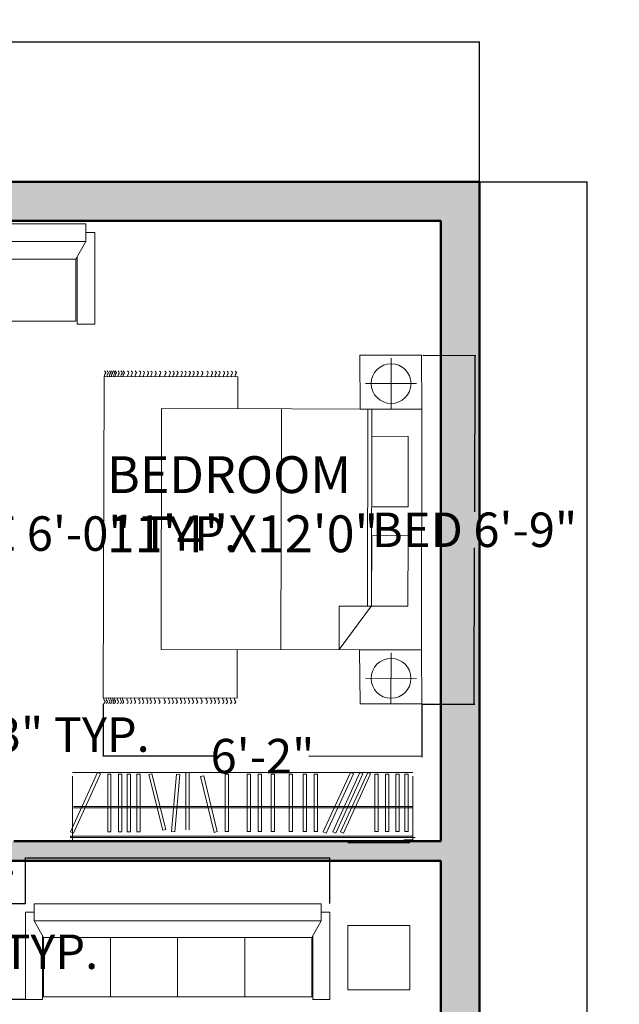
# Model space of a CAD drawing. Units: inches. Extents: x 22042254 to 25404563, y 17568978 to 17626777.
# Tile 44 of 45: x 22180037 to 22180176, y 17626547 to 17626775. Entities that reach past the tile are written whole.
import ezdxf

# ---------------------------------------------------------------- set-up
doc = ezdxf.new("R2010")
doc.units = ezdxf.units.IN
doc.header["$MEASUREMENT"] = 0
for name, color, linetype, lineweight in [('A-ANNO-DIMS', 2, 'Continuous', 18), ('A-AREA-IDEN', 7, 'Continuous', 18), ('A-WALL-PATT', 244, 'Continuous', 13), ('closet', 252, 'Continuous', 18), ('furniture', 8, 'Continuous', 18), ('walls', 252, 'Continuous', 50)]:
    doc.layers.add(name, color=color, linetype=linetype, lineweight=lineweight)
doc.styles.get("Standard").update_dxf_attribs({"font": 'arial.ttf'})
doc.dimstyles.get("Standard").update_dxf_attribs({"dimtxt": 8, "dimasz": 0.18, "dimexe": 0.18, "dimexo": 0.0625, "dimgap": 0.09, "dimtad": 0, "dimtih": 1, "dimtoh": 1, "dimzin": 0, "dimdsep": 46, "dimlunit": 3, "dimtxsty": 'Standard', "dimcen": 0.09, "dimadec": 0, "dimazin": 0, "dimtfac": 1, "dimtofl": 0, "dimtmove": 0, "dimatfit": 3, "dimfxl": 1, "dimtolj": 1, "dimtzin": 0, "dimarcsym": 0})

# ---------------------------------------------------------------- blocks, each defined once
blk = doc.blocks.new('*D1')
at = {"layer": 'A-ANNO-DIMS', "color": 0, "lineweight": -2, "transparency": 16777216}
for p, q in [((22179783.73, 17626737.84), (22179783.73, 17626770.35)), ((22179783.91, 17626770.17), (22179956.86, 17626770.17)), ((22180143.55, 17626770.17), (22179970.61, 17626770.17)), ((22180143.73, 17626737.84), (22180143.73, 17626770.35))]:
    blk.add_line(p, q, dxfattribs=at)
at = {"layer": 'A-ANNO-DIMS', "color": 0, "transparency": 16777216}
for points in [[(22179783.91, 17626770.2), (22179783.91, 17626770.14), (22179783.73, 17626770.17)], [(22180143.55, 17626770.2), (22180143.55, 17626770.14), (22180143.73, 17626770.17)]]:
    blk.add_solid(points, dxfattribs=at)
at = {"layer": 'Defpoints', "color": 0, "transparency": 16777216}
for p in [(22180143.73, 17626770.17), (22179783.73, 17626737.78), (22180143.73, 17626737.78)]:
    blk.add_point(p, dxfattribs=at)
at = {"layer": 'A-ANNO-DIMS', "color": 0, "transparency": 16777216, "insert": (22179963.73, 17626770.17), "char_height": 8, "attachment_point": 5}
blk.add_mtext("\\A1;30'", dxfattribs=at)
blk = doc.blocks.new('*D2')
at = {"layer": 'A-ANNO-DIMS', "color": 0, "lineweight": -2, "transparency": 16777216}
for p, q in [((22180143.8, 17626737.78), (22180168.82, 17626737.78)), ((22180168.64, 17626737.6), (22180168.64, 17626471.94)), ((22180168.64, 17626197.96), (22180168.64, 17626463.62)), ((22180143.8, 17626197.78), (22180168.82, 17626197.78))]:
    blk.add_line(p, q, dxfattribs=at)
at = {"layer": 'A-ANNO-DIMS', "color": 0, "transparency": 16777216}
for points in [[(22180168.61, 17626737.6), (22180168.67, 17626737.6), (22180168.64, 17626737.78)], [(22180168.61, 17626197.96), (22180168.67, 17626197.96), (22180168.64, 17626197.78)]]:
    blk.add_solid(points, dxfattribs=at)
at = {"layer": 'Defpoints', "color": 0, "transparency": 16777216}
for p in [(22180143.73, 17626737.78), (22180168.64, 17626737.78), (22180143.73, 17626197.78)]:
    blk.add_point(p, dxfattribs=at)
at = {"layer": 'A-ANNO-DIMS', "color": 0, "transparency": 16777216, "insert": (22180168.64, 17626467.78), "char_height": 8, "attachment_point": 5}
blk.add_mtext("\\A1;45'", dxfattribs=at)
blk = doc.blocks.new('FABRIC SOFA 4S')
at = {"layer": 'furniture'}
for p, q in [((3, 54), (34, 54)), ((3, 51), (3, 54)), ((34, 48), (34, 54)), ((0, -51), (0, 51)), ((6, 51), (0, 51)), ((6, -51), (6, 51)), ((12, 47.63), (6, 51)), ((11.14, 48), (34, 48)), ((33, 23.81), (12, 23.81)), ((33, 0), (12, 0)), ((33, -23.81), (12, -23.81)), ((6, -51), (12, -47.63)), ((11.54, -48), (34, -48)), ((34, -48), (34, -54)), ((6, -51), (0, -51)), ((3, -54), (3, -51)), ((3, -54), (34, -54))]:
    blk.add_line(p, q, dxfattribs=at)
blk.add_lwpolyline([(12, -47.63), (12, 47.63), (33, 47.63), (33, -47.63)], close=True, dxfattribs=at)
blk = doc.blocks.new('CARPET')
at = {"layer": 'furniture'}
for p, q in [((-51.53, -98.11), (-51.53, -55.12)), ((-51.53, -55.12), (-41.27, -55.12)), ((36, -55.12), (51.55, -55.12)), ((51.55, -55.12), (51.55, -98.11)), ((51.55, -98.11), (-51.53, -98.11))]:
    blk.add_line(p, q, dxfattribs=at)
for points, knots in [([(-53.37, -55.99), (-53.22, -55.8), (-52.9, -55.41), (-52.34, -55.8), (-51.89, -56.08), (-51.65, -55.91), (-51.53, -55.83)], [0, 0, 0, 0, 0.653278, 1.290138, 1.740457, 2.114451, 2.114451, 2.114451, 2.114451]), ([(-53.37, -57.26), (-53.22, -57.07), (-52.9, -56.67), (-52.34, -57.07), (-51.89, -57.35), (-51.65, -57.17), (-51.53, -57.1)], [0, 0, 0, 0, 0.653278, 1.290138, 1.740457, 2.114451, 2.114451, 2.114451, 2.114451]), ([(53.37, -55.99), (53.22, -55.8), (52.9, -55.41), (52.34, -55.8), (51.89, -56.08), (51.65, -55.91), (51.53, -55.83)], [0, 0, 0, 0, 0.653278, 1.290138, 1.740457, 2.114451, 2.114451, 2.114451, 2.114451]), ([(53.37, -57.26), (53.22, -57.07), (52.9, -56.67), (52.34, -57.07), (51.89, -57.35), (51.65, -57.17), (51.53, -57.1)], [0, 0, 0, 0, 0.653278, 1.290138, 1.740457, 2.114451, 2.114451, 2.114451, 2.114451]), ([(-53.37, -58.59), (-53.22, -58.4), (-52.9, -58.01), (-52.34, -58.4), (-51.89, -58.68), (-51.65, -58.5), (-51.53, -58.43)], [0, 0, 0, 0, 0.653278, 1.290138, 1.740457, 2.114451, 2.114451, 2.114451, 2.114451]), ([(-53.37, -59.78), (-53.22, -59.58), (-52.9, -59.19), (-52.34, -59.58), (-51.89, -59.86), (-51.65, -59.69), (-51.53, -59.61)], [0, 0, 0, 0, 0.653278, 1.290138, 1.740457, 2.114451, 2.114451, 2.114451, 2.114451]), ([(53.37, -58.59), (53.22, -58.4), (52.9, -58.01), (52.34, -58.4), (51.89, -58.68), (51.65, -58.5), (51.53, -58.43)], [0, 0, 0, 0, 0.653278, 1.290138, 1.740457, 2.114451, 2.114451, 2.114451, 2.114451]), ([(53.37, -59.78), (53.22, -59.58), (52.9, -59.19), (52.34, -59.58), (51.89, -59.86), (51.65, -59.69), (51.53, -59.61)], [0, 0, 0, 0, 0.653278, 1.290138, 1.740457, 2.114451, 2.114451, 2.114451, 2.114451]), ([(-53.37, -61.22), (-53.22, -61.02), (-52.9, -60.63), (-52.34, -61.02), (-51.89, -61.3), (-51.65, -61.13), (-51.53, -61.05)], [0, 0, 0, 0, 0.653278, 1.290138, 1.740457, 2.114451, 2.114451, 2.114451, 2.114451]), ([(-53.37, -62.44), (-53.22, -62.25), (-52.9, -61.86), (-52.34, -62.25), (-51.89, -62.53), (-51.65, -62.36), (-51.53, -62.28)], [0, 0, 0, 0, 0.653278, 1.290138, 1.740457, 2.114451, 2.114451, 2.114451, 2.114451]), ([(-53.37, -63.63), (-53.22, -63.43), (-52.9, -63.04), (-52.34, -63.43), (-51.89, -63.72), (-51.65, -63.54), (-51.53, -63.46)], [0, 0, 0, 0, 0.653278, 1.290138, 1.740457, 2.114451, 2.114451, 2.114451, 2.114451]), ([(53.37, -61.22), (53.22, -61.02), (52.9, -60.63), (52.34, -61.02), (51.89, -61.3), (51.65, -61.13), (51.53, -61.05)], [0, 0, 0, 0, 0.653278, 1.290138, 1.740457, 2.114451, 2.114451, 2.114451, 2.114451]), ([(53.37, -62.44), (53.22, -62.25), (52.9, -61.86), (52.34, -62.25), (51.89, -62.53), (51.65, -62.36), (51.53, -62.28)], [0, 0, 0, 0, 0.653278, 1.290138, 1.740457, 2.114451, 2.114451, 2.114451, 2.114451]), ([(53.37, -63.63), (53.22, -63.43), (52.9, -63.04), (52.34, -63.43), (51.89, -63.72), (51.65, -63.54), (51.53, -63.46)], [0, 0, 0, 0, 0.653278, 1.290138, 1.740457, 2.114451, 2.114451, 2.114451, 2.114451]), ([(-53.37, -65.07), (-53.22, -64.87), (-52.9, -64.48), (-52.34, -64.87), (-51.89, -65.15), (-51.65, -64.98), (-51.53, -64.9)], [0, 0, 0, 0, 0.653278, 1.290138, 1.740457, 2.114451, 2.114451, 2.114451, 2.114451]), ([(-53.37, -66.76), (-53.22, -66.56), (-52.9, -66.17), (-52.34, -66.56), (-51.89, -66.84), (-51.65, -66.67), (-51.53, -66.59)], [0, 0, 0, 0, 0.653278, 1.290138, 1.740457, 2.114451, 2.114451, 2.114451, 2.114451]), ([(53.37, -65.07), (53.22, -64.87), (52.9, -64.48), (52.34, -64.87), (51.89, -65.15), (51.65, -64.98), (51.53, -64.9)], [0, 0, 0, 0, 0.653278, 1.290138, 1.740457, 2.114451, 2.114451, 2.114451, 2.114451]), ([(53.37, -66.76), (53.22, -66.56), (52.9, -66.17), (52.34, -66.56), (51.89, -66.84), (51.65, -66.67), (51.53, -66.59)], [0, 0, 0, 0, 0.653278, 1.290138, 1.740457, 2.114451, 2.114451, 2.114451, 2.114451]), ([(-53.37, -68.2), (-53.22, -68), (-52.9, -67.61), (-52.34, -68), (-51.89, -68.28), (-51.65, -68.11), (-51.53, -68.03)], [0, 0, 0, 0, 0.653278, 1.290138, 1.740457, 2.114451, 2.114451, 2.114451, 2.114451]), ([(-53.37, -69.53), (-53.22, -69.33), (-52.9, -68.94), (-52.34, -69.33), (-51.89, -69.61), (-51.65, -69.44), (-51.53, -69.36)], [0, 0, 0, 0, 0.653278, 1.290138, 1.740457, 2.114451, 2.114451, 2.114451, 2.114451]), ([(53.37, -68.2), (53.22, -68), (52.9, -67.61), (52.34, -68), (51.89, -68.28), (51.65, -68.11), (51.53, -68.03)], [0, 0, 0, 0, 0.653278, 1.290138, 1.740457, 2.114451, 2.114451, 2.114451, 2.114451]), ([(53.37, -69.53), (53.22, -69.33), (52.9, -68.94), (52.34, -69.33), (51.89, -69.61), (51.65, -69.44), (51.53, -69.36)], [0, 0, 0, 0, 0.653278, 1.290138, 1.740457, 2.114451, 2.114451, 2.114451, 2.114451]), ([(-53.37, -70.79), (-53.22, -70.6), (-52.9, -70.21), (-52.34, -70.6), (-51.89, -70.88), (-51.65, -70.7), (-51.53, -70.63)], [0, 0, 0, 0, 0.653278, 1.290138, 1.740457, 2.114451, 2.114451, 2.114451, 2.114451]), ([(-53.37, -72.12), (-53.22, -71.93), (-52.9, -71.54), (-52.34, -71.93), (-51.89, -72.21), (-51.65, -72.04), (-51.53, -71.96)], [0, 0, 0, 0, 0.653278, 1.290138, 1.740457, 2.114451, 2.114451, 2.114451, 2.114451]), ([(53.37, -70.79), (53.22, -70.6), (52.9, -70.21), (52.34, -70.6), (51.89, -70.88), (51.65, -70.7), (51.53, -70.63)], [0, 0, 0, 0, 0.653278, 1.290138, 1.740457, 2.114451, 2.114451, 2.114451, 2.114451]), ([(53.37, -72.12), (53.22, -71.93), (52.9, -71.54), (52.34, -71.93), (51.89, -72.21), (51.65, -72.04), (51.53, -71.96)], [0, 0, 0, 0, 0.653278, 1.290138, 1.740457, 2.114451, 2.114451, 2.114451, 2.114451]), ([(-53.37, -73.31), (-53.22, -73.11), (-52.9, -72.72), (-52.34, -73.11), (-51.89, -73.4), (-51.65, -73.22), (-51.53, -73.14)], [0, 0, 0, 0, 0.653278, 1.290138, 1.740457, 2.114451, 2.114451, 2.114451, 2.114451]), ([(-53.37, -74.75), (-53.22, -74.55), (-52.9, -74.16), (-52.34, -74.55), (-51.89, -74.83), (-51.65, -74.66), (-51.53, -74.58)], [0, 0, 0, 0, 0.653278, 1.290138, 1.740457, 2.114451, 2.114451, 2.114451, 2.114451]), ([(-53.37, -75.98), (-53.22, -75.78), (-52.9, -75.39), (-52.34, -75.78), (-51.89, -76.06), (-51.65, -75.89), (-51.53, -75.81)], [0, 0, 0, 0, 0.653278, 1.290138, 1.740457, 2.114451, 2.114451, 2.114451, 2.114451]), ([(53.37, -73.31), (53.22, -73.11), (52.9, -72.72), (52.34, -73.11), (51.89, -73.4), (51.65, -73.22), (51.53, -73.14)], [0, 0, 0, 0, 0.653278, 1.290138, 1.740457, 2.114451, 2.114451, 2.114451, 2.114451]), ([(53.37, -74.75), (53.22, -74.55), (52.9, -74.16), (52.34, -74.55), (51.89, -74.83), (51.65, -74.66), (51.53, -74.58)], [0, 0, 0, 0, 0.653278, 1.290138, 1.740457, 2.114451, 2.114451, 2.114451, 2.114451]), ([(53.37, -75.98), (53.22, -75.78), (52.9, -75.39), (52.34, -75.78), (51.89, -76.06), (51.65, -75.89), (51.53, -75.81)], [0, 0, 0, 0, 0.653278, 1.290138, 1.740457, 2.114451, 2.114451, 2.114451, 2.114451]), ([(-53.37, -77.16), (-53.22, -76.96), (-52.9, -76.57), (-52.34, -76.96), (-51.89, -77.25), (-51.65, -77.07), (-51.53, -76.99)], [0, 0, 0, 0, 0.653278, 1.290138, 1.740457, 2.114451, 2.114451, 2.114451, 2.114451]), ([(-53.37, -78.6), (-53.22, -78.4), (-52.9, -78.01), (-52.34, -78.4), (-51.89, -78.68), (-51.65, -78.51), (-51.53, -78.43)], [0, 0, 0, 0, 0.653278, 1.290138, 1.740457, 2.114451, 2.114451, 2.114451, 2.114451]), ([(53.37, -77.16), (53.22, -76.96), (52.9, -76.57), (52.34, -76.96), (51.89, -77.25), (51.65, -77.07), (51.53, -76.99)], [0, 0, 0, 0, 0.653278, 1.290138, 1.740457, 2.114451, 2.114451, 2.114451, 2.114451]), ([(53.37, -78.6), (53.22, -78.4), (52.9, -78.01), (52.34, -78.4), (51.89, -78.68), (51.65, -78.51), (51.53, -78.43)], [0, 0, 0, 0, 0.653278, 1.290138, 1.740457, 2.114451, 2.114451, 2.114451, 2.114451]), ([(-53.37, -80.29), (-53.22, -80.09), (-52.9, -79.7), (-52.34, -80.09), (-51.89, -80.37), (-51.65, -80.2), (-51.53, -80.12)], [0, 0, 0, 0, 0.653278, 1.290138, 1.740457, 2.114451, 2.114451, 2.114451, 2.114451]), ([(-53.37, -81.73), (-53.22, -81.53), (-52.9, -81.14), (-52.34, -81.53), (-51.89, -81.81), (-51.65, -81.64), (-51.53, -81.56)], [0, 0, 0, 0, 0.653278, 1.290138, 1.740457, 2.114451, 2.114451, 2.114451, 2.114451]), ([(53.37, -80.29), (53.22, -80.09), (52.9, -79.7), (52.34, -80.09), (51.89, -80.37), (51.65, -80.2), (51.53, -80.12)], [0, 0, 0, 0, 0.653278, 1.290138, 1.740457, 2.114451, 2.114451, 2.114451, 2.114451]), ([(53.37, -81.73), (53.22, -81.53), (52.9, -81.14), (52.34, -81.53), (51.89, -81.81), (51.65, -81.64), (51.53, -81.56)], [0, 0, 0, 0, 0.653278, 1.290138, 1.740457, 2.114451, 2.114451, 2.114451, 2.114451]), ([(-53.37, -83.06), (-53.22, -82.86), (-52.9, -82.47), (-52.34, -82.86), (-51.89, -83.14), (-51.65, -82.97), (-51.53, -82.89)], [0, 0, 0, 0, 0.653278, 1.290138, 1.740457, 2.114451, 2.114451, 2.114451, 2.114451]), ([(-53.37, -84.18), (-53.22, -83.99), (-52.9, -83.6), (-52.34, -83.99), (-51.89, -84.27), (-51.65, -84.09), (-51.53, -84.02)], [0, 0, 0, 0, 0.653278, 1.290138, 1.740457, 2.114451, 2.114451, 2.114451, 2.114451]), ([(-53.37, -85.51), (-53.22, -85.32), (-52.9, -84.93), (-52.34, -85.32), (-51.89, -85.6), (-51.65, -85.42), (-51.53, -85.35)], [0, 0, 0, 0, 0.653278, 1.290138, 1.740457, 2.114451, 2.114451, 2.114451, 2.114451]), ([(53.37, -83.06), (53.22, -82.86), (52.9, -82.47), (52.34, -82.86), (51.89, -83.14), (51.65, -82.97), (51.53, -82.89)], [0, 0, 0, 0, 0.653278, 1.290138, 1.740457, 2.114451, 2.114451, 2.114451, 2.114451]), ([(53.37, -84.18), (53.22, -83.99), (52.9, -83.6), (52.34, -83.99), (51.89, -84.27), (51.65, -84.09), (51.53, -84.02)], [0, 0, 0, 0, 0.653278, 1.290138, 1.740457, 2.114451, 2.114451, 2.114451, 2.114451]), ([(53.37, -85.51), (53.22, -85.32), (52.9, -84.93), (52.34, -85.32), (51.89, -85.6), (51.65, -85.42), (51.53, -85.35)], [0, 0, 0, 0, 0.653278, 1.290138, 1.740457, 2.114451, 2.114451, 2.114451, 2.114451]), ([(-53.37, -86.7), (-53.22, -86.5), (-52.9, -86.11), (-52.34, -86.5), (-51.89, -86.78), (-51.65, -86.61), (-51.53, -86.53)], [0, 0, 0, 0, 0.653278, 1.290138, 1.740457, 2.114451, 2.114451, 2.114451, 2.114451]), ([(-53.37, -88.14), (-53.22, -87.94), (-52.9, -87.55), (-52.34, -87.94), (-51.89, -88.22), (-51.65, -88.05), (-51.53, -87.97)], [0, 0, 0, 0, 0.653278, 1.290138, 1.740457, 2.114451, 2.114451, 2.114451, 2.114451]), ([(53.37, -86.7), (53.22, -86.5), (52.9, -86.11), (52.34, -86.5), (51.89, -86.78), (51.65, -86.61), (51.53, -86.53)], [0, 0, 0, 0, 0.653278, 1.290138, 1.740457, 2.114451, 2.114451, 2.114451, 2.114451]), ([(53.37, -88.14), (53.22, -87.94), (52.9, -87.55), (52.34, -87.94), (51.89, -88.22), (51.65, -88.05), (51.53, -87.97)], [0, 0, 0, 0, 0.653278, 1.290138, 1.740457, 2.114451, 2.114451, 2.114451, 2.114451]), ([(-53.37, -89.36), (-53.22, -89.17), (-52.9, -88.78), (-52.34, -89.17), (-51.89, -89.45), (-51.65, -89.28), (-51.53, -89.2)], [0, 0, 0, 0, 0.653278, 1.290138, 1.740457, 2.114451, 2.114451, 2.114451, 2.114451]), ([(-53.37, -90.55), (-53.22, -90.35), (-52.9, -89.96), (-52.34, -90.35), (-51.89, -90.64), (-51.65, -90.46), (-51.53, -90.38)], [0, 0, 0, 0, 0.653278, 1.290138, 1.740457, 2.114451, 2.114451, 2.114451, 2.114451]), ([(-53.37, -91.99), (-53.22, -91.79), (-52.9, -91.4), (-52.34, -91.79), (-51.89, -92.07), (-51.65, -91.9), (-51.53, -91.82)], [0, 0, 0, 0, 0.653278, 1.290138, 1.740457, 2.114451, 2.114451, 2.114451, 2.114451]), ([(53.37, -89.36), (53.22, -89.17), (52.9, -88.78), (52.34, -89.17), (51.89, -89.45), (51.65, -89.28), (51.53, -89.2)], [0, 0, 0, 0, 0.653278, 1.290138, 1.740457, 2.114451, 2.114451, 2.114451, 2.114451]), ([(53.37, -90.55), (53.22, -90.35), (52.9, -89.96), (52.34, -90.35), (51.9, -90.63), (51.66, -90.47), (51.55, -90.4)], [0, 0, 0, 0, 0.653278, 1.290138, 1.740457, 2.0926, 2.0926, 2.0926, 2.0926]), ([(53.37, -91.99), (53.22, -91.79), (52.9, -91.4), (52.34, -91.79), (51.9, -92.07), (51.66, -91.91), (51.55, -91.83)], [0, 0, 0, 0, 0.653278, 1.290138, 1.740457, 2.0926, 2.0926, 2.0926, 2.0926]), ([(-53.37, -92.69), (-53.22, -92.48), (-52.9, -92.08), (-52.35, -92.49), (-51.89, -92.77), (-51.65, -92.6), (-51.53, -92.52)], [0, 0, 0, 0, 0.663904, 1.307406, 1.757725, 2.131719, 2.131719, 2.131719, 2.131719]), ([(-53.37, -93.61), (-53.22, -93.42), (-52.9, -93.03), (-52.34, -93.42), (-51.89, -93.7), (-51.65, -93.52), (-51.53, -93.45)], [0, 0, 0, 0, 0.653278, 1.290138, 1.740457, 2.114451, 2.114451, 2.114451, 2.114451]), ([(-53.37, -94.55), (-53.22, -94.35), (-52.9, -93.96), (-52.34, -94.35), (-51.89, -94.63), (-51.65, -94.46), (-51.53, -94.38)], [0, 0, 0, 0, 0.653278, 1.290138, 1.740457, 2.114451, 2.114451, 2.114451, 2.114451]), ([(-53.37, -95.05), (-53.22, -94.85), (-52.9, -94.46), (-52.34, -94.85), (-51.89, -95.14), (-51.65, -94.96), (-51.53, -94.88)], [0, 0, 0, 0, 0.653278, 1.290138, 1.740457, 2.114451, 2.114451, 2.114451, 2.114451]), ([(53.37, -92.69), (53.22, -92.49), (52.9, -92.09), (52.34, -92.49), (51.9, -92.77), (51.66, -92.61), (51.55, -92.53)], [0, 0, 0, 0, 0.656792, 1.295826, 1.746145, 2.098292, 2.098292, 2.098292, 2.098292]), ([(53.37, -93.66), (53.22, -93.46), (52.9, -93.07), (52.34, -93.46), (51.9, -93.74), (51.66, -93.58), (51.55, -93.5)], [0, 0, 0, 0, 0.653278, 1.290138, 1.740457, 2.0926, 2.0926, 2.0926, 2.0926]), ([(53.37, -94.59), (53.22, -94.4), (52.9, -94.01), (52.34, -94.4), (51.9, -94.68), (51.66, -94.51), (51.55, -94.44)], [0, 0, 0, 0, 0.653278, 1.290138, 1.740457, 2.0926, 2.0926, 2.0926, 2.0926]), ([(53.37, -95.1), (53.22, -94.9), (52.9, -94.51), (52.34, -94.9), (51.9, -95.18), (51.66, -95.02), (51.55, -94.94)], [0, 0, 0, 0, 0.653278, 1.290138, 1.740457, 2.0926, 2.0926, 2.0926, 2.0926]), ([(-53.37, -95.73), (-53.22, -95.54), (-52.9, -95.15), (-52.34, -95.54), (-51.89, -95.82), (-51.65, -95.65), (-51.53, -95.57)], [0, 0, 0, 0, 0.653278, 1.290138, 1.740457, 2.114451, 2.114451, 2.114451, 2.114451]), ([(-53.37, -96.38), (-53.22, -96.18), (-52.9, -95.79), (-52.34, -96.18), (-51.89, -96.47), (-51.65, -96.29), (-51.53, -96.21)], [0, 0, 0, 0, 0.653278, 1.290138, 1.740457, 2.114451, 2.114451, 2.114451, 2.114451]), ([(-53.37, -97.17), (-53.22, -96.98), (-52.9, -96.59), (-52.34, -96.98), (-51.89, -97.26), (-51.65, -97.08), (-51.53, -97.01)], [0, 0, 0, 0, 0.653278, 1.290138, 1.740457, 2.114451, 2.114451, 2.114451, 2.114451]), ([(-53.37, -97.99), (-53.22, -97.79), (-52.9, -97.4), (-52.34, -97.79), (-51.89, -98.08), (-51.65, -97.9), (-51.53, -97.82)], [0, 0, 0, 0, 0.653278, 1.290138, 1.740457, 2.114451, 2.114451, 2.114451, 2.114451]), ([(53.37, -95.78), (53.22, -95.58), (52.9, -95.19), (52.34, -95.58), (51.89, -95.86), (51.65, -95.69), (51.53, -95.61)], [0, 0, 0, 0, 0.653278, 1.290138, 1.740457, 2.114451, 2.114451, 2.114451, 2.114451]), ([(53.37, -96.43), (53.22, -96.23), (52.9, -95.84), (52.34, -96.23), (51.89, -96.51), (51.65, -96.34), (51.53, -96.26)], [0, 0, 0, 0, 0.653278, 1.290138, 1.740457, 2.114451, 2.114451, 2.114451, 2.114451]), ([(53.37, -97.22), (53.22, -97.02), (52.9, -96.63), (52.34, -97.02), (51.89, -97.3), (51.65, -97.13), (51.53, -97.05)], [0, 0, 0, 0, 0.653278, 1.290138, 1.740457, 2.114451, 2.114451, 2.114451, 2.114451]), ([(53.37, -97.99), (53.22, -97.79), (52.9, -97.4), (52.34, -97.79), (51.89, -98.08), (51.65, -97.9), (51.53, -97.82)], [0, 0, 0, 0, 0.653278, 1.290138, 1.740457, 2.114451, 2.114451, 2.114451, 2.114451])]:
    blk.add_open_spline(points, degree=3, knots=knots, dxfattribs=at)
blk = doc.blocks.new('A$C58D270C6')
at = {"layer": 'furniture'}
for p, q in [((9.09, 124.13), (9.09, 108.87)), ((1.46, 116.5), (16.73, 116.5)), ((14.97, 94.84), (24.62, 107.92)), ((24.62, 94.93), (24.62, 107.92)), ((42.08, 108), (42.08, 36)), ((14.97, 94.93), (24.62, 94.93)), ((14.97, 94.84), (14.97, 36)), ((16.22, 94.93), (16.22, 36)), ((9.25, 36), (9.25, 20.74)), ((1.62, 28.37), (16.88, 28.37))]:
    blk.add_line(p, q, dxfattribs=at)
for points in [[(18.5, 108), (18.34, 124.13), (-0.16, 124.13), (0, 108)], [(0, 108), (77.91, 108), (77.91, 36), (0, 36)], [(4.09, 94.93), (14.97, 94.93), (14.97, 73.83), (4.09, 73.83)], [(4.09, 65.23), (14.97, 65.23), (14.97, 44.13), (4.09, 44.13)], [(18.65, 19.87), (18.5, 36), (0, 36), (0.16, 19.87)]]:
    blk.add_lwpolyline(points, close=True, dxfattribs=at)
for centre in [(9.09, 116.5), (9.25, 28.37)]:
    blk.add_circle(centre, 5.95, dxfattribs=at)
at = {"layer": 'furniture', "xscale": 0.9312884925094044, "yscale": 0.9312884925094044, "zscale": 0.9312884925094044, "rotation": 90}
blk.add_blockref('CARPET', (3.79, 74.47), dxfattribs=at)
blk = doc.blocks.new('closet')
at = {"layer": 'closet'}
for p, q in [((-0.71, -5.58), (5.59, 8.19)), ((-0.23, 7.39), (-0.23, -6.57)), ((6.27, 7.88), (-0.04, -5.89)), ((5.59, 8.19), (6.27, 7.88)), ((7.92, 7.84), (8.68, 7.84)), ((7.92, 7.84), (7.92, -5.51)), ((8.68, 7.84), (8.68, -5.51)), ((10.44, 7.84), (11.2, 7.84)), ((10.44, 7.84), (10.44, -5.51)), ((11.2, 7.84), (11.2, -5.51)), ((12.45, 7.84), (13.21, 7.84)), ((12.45, 7.84), (12.45, -5.51)), ((13.21, 7.84), (13.21, -5.51)), ((14.71, 7.84), (15.47, 7.84)), ((14.71, 7.84), (14.71, -5.51)), ((15.47, 7.84), (15.47, -5.51)), ((17.44, 7.75), (18.17, 7.93)), ((17.44, 7.75), (20.73, -5.2)), ((18.17, 7.93), (21.46, -5.01)), ((23.92, 7.84), (22.75, -5.46)), ((24.67, 7.78), (23.51, -5.53)), ((23.92, 7.84), (24.67, 7.78)), ((26.09, 8.25), (26.09, -5.1)), ((26.84, 8.25), (26.84, -5.1)), ((29.49, 7.29), (32.64, -5.69)), ((30.22, 7.46), (33.37, -5.51)), ((35.23, 7.84), (35.23, -5.51)), ((35.99, 7.84), (35.99, -5.51)), ((40.33, 7.84), (40.33, -5.51)), ((41.08, 7.84), (41.08, -5.51)), ((42.85, 7.84), (42.85, -5.51)), ((43.61, 7.84), (43.61, -5.51)), ((45.9, 7.84), (45.9, -5.51)), ((46.65, 7.84), (46.65, -5.51)), ((50.07, 7.84), (50.07, -5.51)), ((50.82, 7.84), (50.82, -5.51)), ((53.32, 7.84), (53.32, -5.51)), ((54.08, 7.84), (54.08, -5.51)), ((55.9, 7.84), (55.9, -5.51)), ((56.65, 7.84), (56.65, -5.51)), ((57.99, -5.58), (64.3, 8.19)), ((64.97, 7.88), (58.67, -5.89)), ((60.19, -5.58), (66.49, 8.19)), ((67.17, 7.88), (60.87, -5.89)), ((62, -5.58), (68.3, 8.19)), ((68.98, 7.88), (62.67, -5.89)), ((69.96, 7.84), (69.96, -5.51)), ((70.72, 7.84), (70.72, -5.51)), ((72.43, 7.84), (72.43, -5.51)), ((73.19, 7.84), (73.19, -5.51)), ((74.82, 7.84), (74.82, -5.51)), ((75.57, 7.84), (75.57, -5.51)), ((76.94, 7.84), (76.94, -5.51)), ((77.69, 7.84), (77.69, -5.51)), ((56.23, 0.33), (0, 0.33)), ((56.2, 0), (0, 0)), ((56.2, 0), (78.76, 0)), ((56.23, 0.33), (78.76, 0.33)), ((-0.04, -5.89), (-0.71, -5.58)), ((21.46, -5.01), (20.73, -5.2)), ((23.51, -5.53), (22.75, -5.46)), ((33.37, -5.51), (32.64, -5.69)), ((35.99, -5.51), (35.23, -5.51)), ((41.08, -5.51), (40.33, -5.51)), ((43.61, -5.51), (42.85, -5.51)), ((46.65, -5.51), (45.9, -5.51)), ((50.82, -5.51), (50.07, -5.51)), ((54.08, -5.51), (53.32, -5.51)), ((56.65, -5.51), (55.9, -5.51)), ((58.67, -5.89), (57.99, -5.58)), ((60.87, -5.89), (60.19, -5.58)), ((62.67, -5.89), (62, -5.58)), ((70.72, -5.51), (69.96, -5.51)), ((73.19, -5.51), (72.43, -5.51)), ((75.57, -5.51), (74.82, -5.51)), ((77.69, -5.51), (76.94, -5.51))]:
    blk.add_line(p, q, dxfattribs=at)
blk = doc.blocks.new('rotated closet')
at = {"layer": 'closet'}
for p, q in [((26.32, 0.86), (27.07, 0.86)), ((29.72, -0.11), (30.45, 0.07)), ((35.46, 0.45), (36.22, 0.45)), ((40.56, 0.45), (41.31, 0.45)), ((43.08, 0.45), (43.84, 0.45)), ((46.13, 0.45), (46.88, 0.45)), ((50.3, 0.45), (51.05, 0.45)), ((53.56, 0.45), (54.31, 0.45)), ((56.13, 0.45), (56.88, 0.45)), ((64.53, 0.8), (65.2, 0.49)), ((66.72, 0.8), (67.4, 0.49)), ((68.53, 0.8), (69.21, 0.49)), ((70.19, 0.45), (70.95, 0.45)), ((72.66, 0.45), (73.42, 0.45)), ((75.05, 0.45), (75.81, 0.45)), ((77.17, 0.45), (77.92, 0.45)), ((78.99, 0), (78.99, -13.96)), ((8.91, -12.91), (8.15, -12.91)), ((11.43, -12.91), (10.67, -12.91)), ((13.44, -12.91), (12.68, -12.91)), ((15.7, -12.91), (14.94, -12.91)), ((-0.46, -14.27), (79.54, -14.27)), ((0, -13.96), (78.99, -13.96))]:
    blk.add_line(p, q, dxfattribs=at)
blk.add_blockref('closet', (0.23, -7.39), dxfattribs=at)
blk = doc.blocks.new('FABRIC SOFA 1S')
at = {"layer": 'furniture'}
for p, q in [((3, 18.12), (34, 18.12)), ((3, 15.12), (3, 18.12)), ((34, 12.12), (34, 18.12)), ((0, -15.12), (0, 15.12)), ((6, 15.12), (0, 15.12)), ((6, -15.12), (6, 15.12)), ((12, 11.75), (6, 15.12)), ((11.33, 12.12), (34, 12.12)), ((6, -15.12), (12, -11.75)), ((11.33, -12.12), (34, -12.12)), ((34, -12.12), (34, -18.12)), ((6, -15.12), (0, -15.12)), ((3, -18.12), (3, -15.12)), ((3, -18.12), (34, -18.12))]:
    blk.add_line(p, q, dxfattribs=at)
blk.add_lwpolyline([(12, -11.75), (12, 11.75), (33, 11.75), (33, -11.75)], close=True, dxfattribs=at)
blk = doc.blocks.new('END-TABLE')
for p, q in [((0, 0), (0, 14.95)), ((0, 14.95), (14.41, 14.95)), ((14.41, 14.95), (14.41, 0)), ((0, 0), (14.41, 0))]:
    blk.add_line(p, q)
blk = doc.blocks.new('*D34')
at = {"layer": 'A-ANNO-DIMS', "color": 0, "lineweight": -2, "transparency": 16777216}
for p, q in [((22180130.61, 17626697.57), (22180142.87, 17626697.54)), ((22180142.69, 17626697.36), (22180142.61, 17626661.24)), ((22180142.51, 17626616.77), (22180142.59, 17626652.89)), ((22180130.43, 17626616.62), (22180142.69, 17626616.59))]:
    blk.add_line(p, q, dxfattribs=at)
at = {"layer": 'A-ANNO-DIMS', "color": 0, "transparency": 16777216}
for points in [[(22180142.66, 17626697.36), (22180142.72, 17626697.36), (22180142.69, 17626697.54)], [(22180142.48, 17626616.77), (22180142.54, 17626616.77), (22180142.51, 17626616.59)]]:
    blk.add_solid(points, dxfattribs=at)
at = {"layer": 'Defpoints', "color": 0, "transparency": 16777216}
for p in [(22180130.54, 17626697.57), (22180130.37, 17626616.62), (22180142.51, 17626616.59)]:
    blk.add_point(p, dxfattribs=at)
at = {"layer": 'A-ANNO-DIMS', "color": 0, "transparency": 16777216, "insert": (22180142.6, 17626657.07), "char_height": 8, "attachment_point": 5}
blk.add_mtext('\\A1;BED 6\'-9"', dxfattribs=at)
blk = doc.blocks.new('*D35')
at = {"layer": 'A-ANNO-DIMS', "color": 0, "lineweight": -2, "transparency": 16777216}
for p, q in [((22180056.4, 17626616.71), (22180056.37, 17626604.45)), ((22180130.37, 17626616.55), (22180130.34, 17626604.29)), ((22180056.55, 17626604.63), (22180082.61, 17626604.58)), ((22180130.16, 17626604.47), (22180104.1, 17626604.53))]:
    blk.add_line(p, q, dxfattribs=at)
at = {"layer": 'A-ANNO-DIMS', "color": 0, "transparency": 16777216}
for points in [[(22180056.55, 17626604.66), (22180056.55, 17626604.6), (22180056.37, 17626604.63)], [(22180130.16, 17626604.5), (22180130.16, 17626604.44), (22180130.34, 17626604.47)]]:
    blk.add_solid(points, dxfattribs=at)
at = {"layer": 'Defpoints', "color": 0, "transparency": 16777216}
for p in [(22180056.4, 17626616.77), (22180130.37, 17626616.62), (22180056.37, 17626604.63)]:
    blk.add_point(p, dxfattribs=at)
at = {"layer": 'A-ANNO-DIMS', "color": 0, "transparency": 16777216, "insert": (22180093.36, 17626604.55), "char_height": 8, "attachment_point": 5}
blk.add_mtext('\\A1;6\'-2"', dxfattribs=at)
blk = doc.blocks.new('*D38')
at = {"layer": 'A-ANNO-DIMS', "color": 0, "lineweight": -2, "transparency": 16777216}
for p, q in [((22180018.54, 17626692.07), (22180029.42, 17626692.07)), ((22180029.24, 17626691.89), (22180029.24, 17626660.42)), ((22180029.24, 17626620.49), (22180029.24, 17626651.96)), ((22180018.54, 17626620.31), (22180029.42, 17626620.31))]:
    blk.add_line(p, q, dxfattribs=at)
at = {"layer": 'A-ANNO-DIMS', "color": 0, "transparency": 16777216}
for points in [[(22180029.21, 17626691.89), (22180029.27, 17626691.89), (22180029.24, 17626692.07)], [(22180029.21, 17626620.49), (22180029.27, 17626620.49), (22180029.24, 17626620.31)]]:
    blk.add_solid(points, dxfattribs=at)
at = {"layer": 'Defpoints', "color": 0, "transparency": 16777216}
for p in [(22180018.48, 17626692.07), (22180029.24, 17626692.07), (22180018.48, 17626620.31)]:
    blk.add_point(p, dxfattribs=at)
at = {"layer": 'A-ANNO-DIMS', "color": 0, "transparency": 16777216, "insert": (22180029.24, 17626656.19), "char_height": 8, "attachment_point": 5}
blk.add_mtext('\\A1;TV CONSOLE 6\'-0" TYP.', dxfattribs=at)
blk = doc.blocks.new('*D39')
at = {"layer": 'A-ANNO-DIMS', "color": 0, "lineweight": -2, "transparency": 16777216}
for p, q in [((22180003.26, 17626620.25), (22180003.26, 17626609.36)), ((22180018.48, 17626620.25), (22180018.48, 17626609.36)), ((22180003.44, 17626609.54), (22180018.3, 17626609.54)), ((22180018.48, 17626609.54), (22180018.66, 17626609.54))]:
    blk.add_line(p, q, dxfattribs=at)
at = {"layer": 'A-ANNO-DIMS', "color": 0, "transparency": 16777216}
for points in [[(22180003.44, 17626609.57), (22180003.44, 17626609.51), (22180003.26, 17626609.54)], [(22180018.3, 17626609.57), (22180018.3, 17626609.51), (22180018.48, 17626609.54)]]:
    blk.add_solid(points, dxfattribs=at)
at = {"layer": 'Defpoints', "color": 0, "transparency": 16777216}
for p in [(22180003.26, 17626620.31), (22180018.48, 17626620.31), (22180018.48, 17626609.54)]:
    blk.add_point(p, dxfattribs=at)
at = {"layer": 'A-ANNO-DIMS', "color": 0, "transparency": 16777216, "insert": (22180042.75, 17626609.54), "char_height": 8, "attachment_point": 5}
blk.add_mtext('\\A1;1\'-3" TYP.', dxfattribs=at)
blk = doc.blocks.new('*D48')
at = {"layer": 'A-ANNO-DIMS', "color": 0, "lineweight": -2, "transparency": 16777216}
for p, q in [((22180038.35, 17626580.87), (22180038.17, 17626580.87)), ((22180038.35, 17626570.34), (22180038.35, 17626581.05)), ((22180108.78, 17626580.87), (22180038.53, 17626580.87)), ((22180108.96, 17626570.34), (22180108.96, 17626581.05))]:
    blk.add_line(p, q, dxfattribs=at)
at = {"layer": 'A-ANNO-DIMS', "color": 0, "transparency": 16777216}
for points in [[(22180038.53, 17626580.9), (22180038.53, 17626580.84), (22180038.35, 17626580.87)], [(22180108.78, 17626580.9), (22180108.78, 17626580.84), (22180108.96, 17626580.87)]]:
    blk.add_solid(points, dxfattribs=at)
at = {"layer": 'Defpoints', "color": 0, "transparency": 16777216}
for p in [(22180038.35, 17626580.87), (22180038.35, 17626570.27), (22180108.96, 17626570.27)]:
    blk.add_point(p, dxfattribs=at)
at = {"layer": 'A-ANNO-DIMS', "color": 0, "transparency": 16777216, "insert": (22179984.52, 17626580.87), "char_height": 8, "attachment_point": 5}
blk.add_mtext('\\A1;SOFA 5\'-10 1/2" TYP.', dxfattribs=at)
blk = doc.blocks.new('*D49')
at = {"layer": 'A-ANNO-DIMS', "color": 0, "lineweight": -2, "transparency": 16777216}
for p, q in [((22180038.29, 17626570.27), (22180027.58, 17626570.27)), ((22180027.76, 17626570.09), (22180027.76, 17626563.33)), ((22180027.76, 17626548.22), (22180027.76, 17626554.98)), ((22180038.29, 17626548.04), (22180027.58, 17626548.04))]:
    blk.add_line(p, q, dxfattribs=at)
at = {"layer": 'A-ANNO-DIMS', "color": 0, "transparency": 16777216}
for points in [[(22180027.73, 17626570.09), (22180027.79, 17626570.09), (22180027.76, 17626570.27)], [(22180027.73, 17626548.22), (22180027.79, 17626548.22), (22180027.76, 17626548.04)]]:
    blk.add_solid(points, dxfattribs=at)
at = {"layer": 'Defpoints', "color": 0, "transparency": 16777216}
for p in [(22180038.35, 17626570.27), (22180027.76, 17626548.04), (22180038.35, 17626548.04)]:
    blk.add_point(p, dxfattribs=at)
at = {"layer": 'A-ANNO-DIMS', "color": 0, "transparency": 16777216, "insert": (22180027.76, 17626559.16), "char_height": 8, "attachment_point": 5}
blk.add_mtext('\\A1;1\'-10" TYP.', dxfattribs=at)

msp = doc.modelspace()

# ---------------------------------------------------------------- hatches: boundary and pattern name
at = {"layer": 'A-WALL-PATT'}
h = msp.add_hatch(color=256, dxfattribs=at)
h.dxf.hatch_style = 1
h.paths.add_polyline_path([(22179792.734, 17626580.28), (22179888.734, 17626580.28), (22179888.734, 17626559.623), (22179893.234, 17626559.623), (22179893.234, 17626580.28), (22179900.438, 17626580.28), (22179900.438, 17626584.78), (22179792.734, 17626584.78), (22179792.734, 17626728.78), (22180134.734, 17626728.78), (22180134.734, 17626584.78), (22180035.602, 17626584.78), (22180004.432, 17626584.78), (22180001.734, 17626584.78), (22180001.734, 17626580.28), (22180134.734, 17626580.28), (22180134.734, 17626404.28), (22180064.487, 17626404.28), (22180064.487, 17626399.78), (22180134.734, 17626399.78), (22180134.734, 17626197.78), (22180143.734, 17626197.78), (22180143.734, 17626737.78), (22179783.734, 17626737.78), (22179783.734, 17626197.78), (22179792.734, 17626197.78), (22179792.734, 17626394.78), (22179936.734, 17626394.78), (22179936.734, 17626383.208), (22179941.234, 17626383.208), (22179941.234, 17626532.28), (22179927.066, 17626532.28), (22179927.066, 17626527.78), (22179928.072, 17626527.78), (22179936.734, 17626527.78), (22179936.734, 17626403.78), (22179792.734, 17626403.78), (22179792.734, 17626527.78), (22179905.094, 17626527.78), (22179905.094, 17626532.28), (22179792.734, 17626532.28)])
h = msp.add_hatch(color=256, dxfattribs=at)
h.dxf.hatch_style = 1
h.paths.add_polyline_path([(22179941.234, 17626336.599), (22179936.734, 17626336.599), (22179936.734, 17626270.28), (22180065.734, 17626270.28), (22180065.734, 17626197.78), (22180074.734, 17626197.78), (22180074.734, 17626279.28), (22180025.734, 17626279.28), (22180025.734, 17626404.28), (22180021.234, 17626404.28), (22180021.234, 17626279.28), (22179941.234, 17626279.28), (22179941.234, 17626327.28), (22179991.805, 17626327.28), (22179991.805, 17626331.78), (22179941.234, 17626331.78)])
h.paths.add_polyline_path([(22180036.005, 17626206.78), (22179936.734, 17626206.78), (22179936.734, 17626197.78), (22180036.005, 17626197.78)], flags=17)
h.paths.add_polyline_path([(22179836.995, 17626451.976), (22179902.189, 17626451.976), (22179902.189, 17626465.064), (22179836.995, 17626465.064)], flags=9)
h.paths.add_polyline_path([(22179836.966, 17626465.674), (22179903.069, 17626465.674), (22179903.069, 17626478.937), (22179836.966, 17626478.937)], flags=9)
h.paths.add_polyline_path([(22180055.036, 17626649.533), (22180120.23, 17626649.533), (22180120.23, 17626662.622), (22180055.036, 17626662.622)], flags=9)
h.paths.add_polyline_path([(22180055.007, 17626663.231), (22180121.111, 17626663.231), (22180121.111, 17626676.495), (22180055.007, 17626676.495)], flags=9)

# ---------------------------------------------------------------- linework, layer by layer
at = {"layer": 'closet'}
for p, q in [((22180128.249, 17626600.773), (22180049.26, 17626600.773)), ((22180049.26, 17626599.905), (22180049.26, 17626585.095)), ((22180128.249, 17626585.095), (22180128.249, 17626599.905)), ((22180048.804, 17626585.963), (22180126.149, 17626585.963)), ((22180048.804, 17626585.648), (22180048.804, 17626585.963)), ((22180048.804, 17626585.963), (22180049.26, 17626585.963)), ((22180048.804, 17626584.78), (22180128.804, 17626584.78)), ((22180126.149, 17626585.095), (22180128.249, 17626585.095)), ((22180126.149, 17626585.095), (22180128.249, 17626585.095))]:
    msp.add_line(p, q, dxfattribs=at)
at = {"layer": 'furniture'}
msp.add_line((22180113.158, 17626584.446), (22180127.568, 17626584.446), dxfattribs=at)
at = {"layer": 'walls'}
for p, q in [((22179783.734, 17626737.78), (22180143.734, 17626737.78)), ((22180143.734, 17626737.78), (22180143.734, 17626197.78)), ((22179792.734, 17626728.78), (22180134.734, 17626728.78)), ((22180134.734, 17626728.78), (22180134.734, 17626584.78)), ((22180035.602, 17626584.78), (22180134.734, 17626584.78)), ((22179893.234, 17626580.28), (22180134.734, 17626580.28)), ((22180134.734, 17626580.28), (22180134.734, 17626404.28))]:
    msp.add_line(p, q, dxfattribs=at)

# ---------------------------------------------------------------- block references
at = {"layer": 'closet'}
msp.add_blockref('rotated closet', (22180049.26, 17626599.923), dxfattribs=at)
at = {"layer": 'furniture'}
for name, p, xscale, yscale, zscale, rotation in [('FABRIC SOFA 1S', (22180041.998, 17626728.088), 0.685544738852578, 0.685544738852578, 0.685544738852578, 270), ('A$C58D270C6', (22180130.455, 17626712.99), 0.7760819264481366, 0.7760819264481366, 0.7760819264481366, 179.8769049998251), ('FABRIC SOFA 4S', (22180073.655, 17626570.274), -0.6537939928824033, 0.6537939928824033, 0.6537939928824033, 89.9999999998931)]:
    msp.add_blockref(name, p, dxfattribs=dict(at, xscale=xscale, yscale=yscale, zscale=zscale, rotation=rotation))
msp.add_blockref('END-TABLE', (22180113.158, 17626550.332), dxfattribs=at)

# ---------------------------------------------------------------- texts
at = {"layer": 'A-AREA-IDEN'}
for s, height, p in [('BEDROOM', 8.5453, (22180057.218, 17626665.587)), ('11\'4"X12\'0"', 8.54529, (22180057.218, 17626651.86))]:
    msp.add_text(s, height=height, dxfattribs=at).set_placement(p)

# ---------------------------------------------------------------- dimensions: what is measured, and where the dimension line sits
at = {"layer": 'A-ANNO-DIMS'}
dim = msp.add_linear_dim(base=(22180143.734, 17626770.174), p1=(22179783.734, 17626737.78), p2=(22180143.734, 17626737.78), dimstyle='Standard', override={"dimclrd": 0, "dimclre": 0, "dimclrt": 0}, dxfattribs=at)
dim.commit()
dim.dimension.update_dxf_attribs({"geometry": '*D1', "text_midpoint": (22179963.734, 17626770.174)})
for base, p1, p2, angle, override, picture, middle in [((22180168.64, 17626737.78), (22180143.734, 17626197.78), (22180143.734, 17626737.78), 90, {"dimclrd": 0, "dimclre": 0, "dimclrt": 0}, '*D2', (22180168.64, 17626467.78)), ((22180056.371, 17626604.631), (22180130.369, 17626616.616), (22180056.398, 17626616.774), 179.87691, {"dimdec": 1, "dimlfac": 1, "dimrnd": 0, "dimzin": 1, "dimdsep": 46, "dimlunit": 4, "dimfrac": 2}, '*D35', (22180093.357, 17626604.552))]:
    dim = msp.add_linear_dim(base=base, p1=p1, p2=p2, angle=angle, dimstyle='Standard', override=override, dxfattribs=at)
    dim.commit()
    dim.dimension.update_dxf_attribs({"geometry": picture, "text_midpoint": middle})
for base, p1, p2, angle, text, picture, middle in [((22180142.512, 17626616.589), (22180130.543, 17626697.569), (22180130.369, 17626616.616), 269.8769, 'BED <>', '*D34', (22180142.599, 17626657.066)), ((22180029.241, 17626692.074), (22180018.476, 17626620.308), (22180018.476, 17626692.074), 90, 'TV CONSOLE <> TYP.', '*D38', (22180029.241, 17626656.191)), ((22180038.35, 17626580.865), (22180108.959, 17626570.274), (22180038.35, 17626570.274), 180, 'SOFA <> TYP.', '*D48', (22179984.522, 17626580.865)), ((22180027.758, 17626548.045), (22180038.35, 17626570.274), (22180038.35, 17626548.045), 270, '<> TYP.', '*D49', (22180027.758, 17626559.159))]:
    dim = msp.add_linear_dim(base=base, p1=p1, p2=p2, angle=angle, text=text, dimstyle='Standard', override={"dimdec": 1, "dimlfac": 1, "dimrnd": 0, "dimzin": 1, "dimdsep": 46, "dimlunit": 4, "dimfrac": 2}, dxfattribs=at)
    dim.commit()
    dim.dimension.update_dxf_attribs({"geometry": picture, "text_midpoint": middle})
dim = msp.add_linear_dim(base=(22180018.476, 17626609.543), p1=(22180003.262, 17626620.308), p2=(22180018.476, 17626620.308), text='<> TYP.', dimstyle='Standard', override={"dimdec": 1, "dimlfac": 1, "dimrnd": 0, "dimzin": 1, "dimdsep": 46, "dimlunit": 4, "dimfrac": 2}, dxfattribs=at)
dim.commit()
dim.dimension.update_dxf_attribs({"geometry": '*D39', "text_midpoint": (22180042.751, 17626609.543)})

doc.saveas('drawing.dxf')
